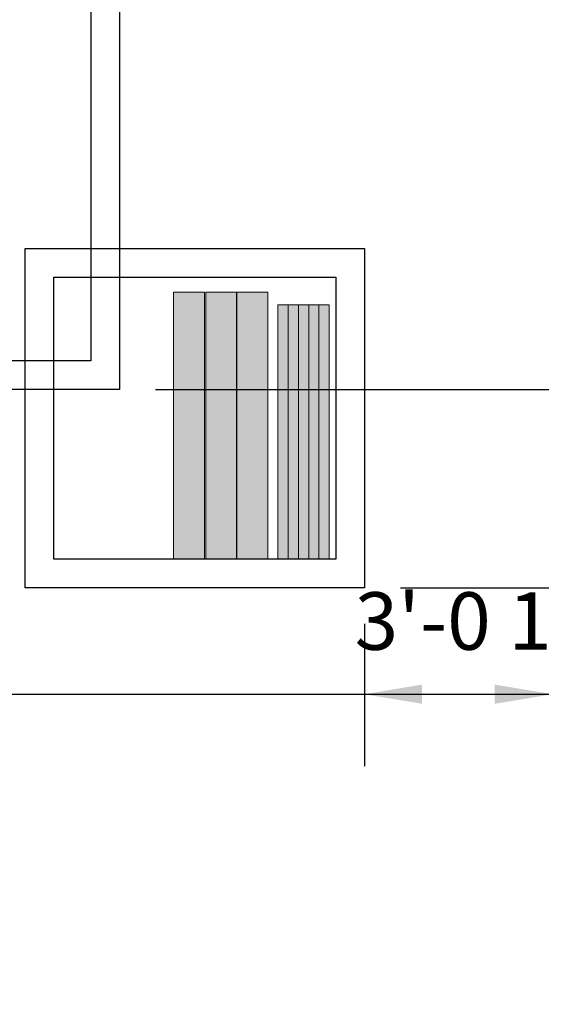
# Model space of a CAD drawing. Units: millimetres. Extents: x 7894 to 8038, y 6851 to 6951.
# Tile 5 of 49: x 7954.15 to 7963.22, y 6854.37 to 6871.49. Entities that reach past the tile are written whole.
import ezdxf

# ---------------------------------------------------------------- set-up
doc = ezdxf.new("R2010")
doc.units = ezdxf.units.MM
for name, color, linetype, lineweight in [('A-ANNO-DIMS', 2, 'Continuous', 18), ('A-FURN-BOOK', 8, 'Continuous', 13), ('A-FURN-CASE', 7, 'Continuous', 30)]:
    doc.layers.add(name, color=color, linetype=linetype, lineweight=lineweight)
doc.layers.add('A-FURN-PATT', color=32, linetype='Continuous', lineweight=9, true_color=0xcd6928)
doc.styles.get("Standard").update_dxf_attribs({"font": 'arial.ttf'})
doc.dimstyles.new('ISO-25', dxfattribs={"dimtxt": 1, "dimasz": 1, "dimexe": 1.25, "dimexo": 0.625, "dimtad": 1, "dimdec": 0, "dimlunit": 4, "dimtxsty": 'Standard', "dimcen": 2.5, "dimclrt": 1, "dimadec": 0, "dimazin": 0, "dimtfac": 1, "dimtdec": 0, "dimtmove": 0, "dimatfit": 3, "dimfxl": 1, "dimarcsym": 0})

# ---------------------------------------------------------------- blocks, each defined once
blk = doc.blocks.new('BOX-SHELF-SMALL-ELEV')
for points in [[(0, 5.9), (5.9, 5.9), (5.9, 0), (0, 0)], [(0.5, 5.4), (5.4, 5.4), (5.4, 0.5), (0.5, 0.5)]]:
    blk.add_lwpolyline(points, close=True)
blk = doc.blocks.new('*D36')
at = {"layer": 'A-ANNO-DIMS', "color": 0, "lineweight": -2, "transparency": 16777216}
for p, q in [((7980.836, 6877.959), (7980.836, 6858.512)), ((7944.487, 6864.436), (7944.487, 6858.512)), ((7945.487, 6859.762), (7979.836, 6859.762))]:
    blk.add_line(p, q, dxfattribs=at)
at = {"layer": 'A-ANNO-DIMS', "color": 0, "transparency": 16777216}
for points in [[(7945.487, 6859.929), (7945.487, 6859.596), (7944.487, 6859.762)], [(7979.836, 6859.929), (7979.836, 6859.596), (7980.836, 6859.762)]]:
    blk.add_solid(points, dxfattribs=at)
at = {"layer": 'Defpoints', "color": 0, "transparency": 16777216}
for p in [(7980.836, 6878.584), (7944.487, 6865.061), (7980.836, 6859.762)]:
    blk.add_point(p, dxfattribs=at)
at = {"layer": 'A-ANNO-DIMS', "color": 1, "transparency": 16777216, "insert": (7962.661, 6860.905), "char_height": 1, "attachment_point": 5}
blk.add_mtext('3\'-0 1/2"', dxfattribs=at)
blk = doc.blocks.new('*D37')
at = {"layer": 'A-ANNO-DIMS', "color": 0, "lineweight": -2, "transparency": 16777216}
for p, q in [((7954.92, 6887.903), (7941.389, 6887.903)), ((7942.639, 6862.61), (7942.639, 6886.903)), ((7953.623, 6861.61), (7941.389, 6861.61))]:
    blk.add_line(p, q, dxfattribs=at)
at = {"layer": 'A-ANNO-DIMS', "color": 0, "transparency": 16777216}
for points in [[(7942.472, 6886.903), (7942.806, 6886.903), (7942.639, 6887.903)], [(7942.472, 6862.61), (7942.806, 6862.61), (7942.639, 6861.61)]]:
    blk.add_solid(points, dxfattribs=at)
at = {"layer": 'Defpoints', "color": 0, "transparency": 16777216}
for p in [(7942.639, 6887.903), (7955.545, 6887.903), (7954.248, 6861.61)]:
    blk.add_point(p, dxfattribs=at)
at = {"layer": 'A-ANNO-DIMS', "color": 1, "transparency": 16777216, "insert": (7941.497, 6874.756), "char_height": 1, "attachment_point": 5, "rotation": 90}
blk.add_mtext('2\'-2 1/2"', dxfattribs=at)
blk = doc.blocks.new('*D41')
at = {"layer": 'A-ANNO-DIMS', "color": 0, "lineweight": -2, "transparency": 16777216}
for p, q in [((7982.683, 6865.722), (7982.683, 6870.631)), ((7964.039, 6864.722), (7983.933, 6864.722)), ((7982.683, 6861.61), (7982.683, 6864.722)), ((7960.773, 6861.61), (7983.933, 6861.61)), ((7982.683, 6860.61), (7982.683, 6859.61))]:
    blk.add_line(p, q, dxfattribs=at)
at = {"layer": 'A-ANNO-DIMS', "color": 0, "transparency": 16777216}
for points in [[(7982.517, 6865.722), (7982.85, 6865.722), (7982.683, 6864.722)], [(7982.517, 6860.61), (7982.85, 6860.61), (7982.683, 6861.61)]]:
    blk.add_solid(points, dxfattribs=at)
at = {"layer": 'Defpoints', "color": 0, "transparency": 16777216}
for p in [(7963.414, 6864.722), (7982.683, 6864.722), (7960.148, 6861.61)]:
    blk.add_point(p, dxfattribs=at)
at = {"layer": 'A-ANNO-DIMS', "color": 1, "transparency": 16777216, "insert": (7981.548, 6868.677), "char_height": 1, "attachment_point": 5, "rotation": 90}
blk.add_mtext('0\'-3"', dxfattribs=at)
blk = doc.blocks.new('*D44')
at = {"layer": 'A-ANNO-DIMS', "color": 0, "lineweight": -2, "transparency": 16777216}
for p, q in [((7963.414, 6864.097), (7963.414, 6858.512)), ((7960.148, 6860.985), (7960.148, 6858.512)), ((7961.148, 6859.762), (7962.414, 6859.762)), ((7963.414, 6859.762), (7970.652, 6859.762))]:
    blk.add_line(p, q, dxfattribs=at)
at = {"layer": 'A-ANNO-DIMS', "color": 0, "transparency": 16777216}
for points in [[(7961.148, 6859.929), (7961.148, 6859.596), (7960.148, 6859.762)], [(7962.414, 6859.929), (7962.414, 6859.596), (7963.414, 6859.762)]]:
    blk.add_solid(points, dxfattribs=at)
at = {"layer": 'Defpoints', "color": 0, "transparency": 16777216}
for p in [(7963.414, 6864.722), (7960.148, 6861.61), (7963.414, 6859.762)]:
    blk.add_point(p, dxfattribs=at)
at = {"layer": 'A-ANNO-DIMS', "color": 1, "transparency": 16777216, "insert": (7967.533, 6860.905), "char_height": 1, "attachment_point": 5}
blk.add_mtext('0\'-3 1/2"', dxfattribs=at)
blk = doc.blocks.new('*D45')
at = {"layer": 'A-ANNO-DIMS', "color": 0, "lineweight": -2, "transparency": 16777216}
for p, q in [((7956.512, 6865.061), (7983.933, 6865.061)), ((7982.683, 6864.061), (7982.683, 6862.61)), ((7960.773, 6861.61), (7983.933, 6861.61)), ((7982.683, 6861.61), (7982.683, 6854.371))]:
    blk.add_line(p, q, dxfattribs=at)
at = {"layer": 'A-ANNO-DIMS', "color": 0, "transparency": 16777216}
for points in [[(7982.517, 6864.061), (7982.85, 6864.061), (7982.683, 6865.061)], [(7982.517, 6862.61), (7982.85, 6862.61), (7982.683, 6861.61)]]:
    blk.add_solid(points, dxfattribs=at)
at = {"layer": 'Defpoints', "color": 0, "transparency": 16777216}
for p in [(7955.887, 6865.061), (7960.148, 6861.61), (7982.683, 6861.61)]:
    blk.add_point(p, dxfattribs=at)
at = {"layer": 'A-ANNO-DIMS', "color": 1, "transparency": 16777216, "insert": (7981.541, 6857.49), "char_height": 1, "attachment_point": 5, "rotation": 90}
blk.add_mtext('0\'-3 1/2"', dxfattribs=at)

msp = doc.modelspace()

# ---------------------------------------------------------------- hatches: boundary and pattern name
at = {"layer": 'A-FURN-PATT'}
h = msp.add_hatch(color=256, dxfattribs=at)
h.dxf.hatch_style = 1
h.paths.add_polyline_path([(7957.367, 6866.754), (7956.826, 6866.754), (7956.826, 6862.11), (7957.367, 6862.11)])
h.paths.add_polyline_path([(7957.925, 6866.754), (7957.386, 6866.754), (7957.386, 6862.11), (7957.925, 6862.11)])
h.paths.add_polyline_path([(7958.465, 6866.754), (7957.926, 6866.754), (7957.926, 6862.11), (7958.466, 6862.11)])
h = msp.add_hatch(color=256, dxfattribs=at)
h.dxf.hatch_style = 1
h.paths.add_polyline_path([(7958.999, 6866.533), (7958.821, 6866.533), (7958.821, 6862.11), (7958.999, 6862.11)])
h.paths.add_polyline_path([(7958.821, 6866.533), (7958.643, 6866.533), (7958.643, 6862.11), (7958.821, 6862.11)])
h = msp.add_hatch(color=256, dxfattribs=at)
h.dxf.hatch_style = 1
h.paths.add_polyline_path([(7959.534, 6866.533), (7959.356, 6866.533), (7959.356, 6862.11), (7959.534, 6862.11)])
h.paths.add_polyline_path([(7959.356, 6866.533), (7959.178, 6866.533), (7959.178, 6862.11), (7959.356, 6862.11)])
h.paths.add_polyline_path([(7959.178, 6866.533), (7958.999, 6866.533), (7958.999, 6862.11), (7959.178, 6862.11)])

# ---------------------------------------------------------------- linework, layer by layer
at = {"layer": 'A-FURN-BOOK'}
for p, q in [((7958.466, 6862.11), (7958.465, 6866.754)), ((7958.643, 6862.11), (7958.643, 6866.533)), ((7958.821, 6866.533), (7958.643, 6866.533)), ((7958.821, 6862.11), (7958.821, 6866.533)), ((7958.999, 6866.533), (7958.821, 6866.533)), ((7958.999, 6862.11), (7958.999, 6866.533)), ((7959.178, 6866.533), (7958.999, 6866.533)), ((7959.178, 6862.11), (7959.178, 6866.533)), ((7959.356, 6866.533), (7959.178, 6866.533)), ((7959.356, 6862.11), (7959.356, 6866.533)), ((7959.534, 6866.533), (7959.356, 6866.533)), ((7959.534, 6862.11), (7959.534, 6866.533)), ((7957.45, 6862.11), (7957.348, 6862.11)), ((7957.553, 6862.11), (7957.45, 6862.11)), ((7957.656, 6862.11), (7957.553, 6862.11)), ((7957.759, 6862.11), (7957.656, 6862.11)), ((7957.861, 6862.11), (7957.759, 6862.11)), ((7957.964, 6862.11), (7957.861, 6862.11)), ((7958.643, 6862.11), (7958.466, 6862.11)), ((7958.821, 6862.11), (7958.643, 6862.11)), ((7958.999, 6862.11), (7958.821, 6862.11)), ((7959.02, 6862.11), (7958.918, 6862.11)), ((7959.178, 6862.11), (7958.999, 6862.11)), ((7959.123, 6862.11), (7959.02, 6862.11)), ((7959.226, 6862.11), (7959.123, 6862.11)), ((7959.356, 6862.11), (7959.178, 6862.11)), ((7959.329, 6862.11), (7959.226, 6862.11)), ((7959.432, 6862.11), (7959.329, 6862.11)), ((7959.534, 6862.11), (7959.356, 6862.11)), ((7959.534, 6862.11), (7959.432, 6862.11))]:
    msp.add_line(p, q, dxfattribs=at)
for points in [[(7956.826, 6866.754), (7957.367, 6866.754), (7957.367, 6862.11), (7956.826, 6862.11)], [(7957.386, 6866.754), (7957.926, 6866.754), (7957.926, 6862.11), (7957.386, 6862.11)], [(7957.925, 6866.754), (7958.466, 6866.754), (7958.466, 6862.11), (7957.925, 6862.11)]]:
    msp.add_lwpolyline(points, close=True, dxfattribs=at)
at = {"layer": 'A-FURN-CASE'}
for points in [[(7944.487, 6876.461), (7955.887, 6876.461), (7955.887, 6865.061), (7944.487, 6865.061)], [(7944.987, 6875.961), (7955.387, 6875.961), (7955.387, 6865.561), (7944.987, 6865.561)]]:
    msp.add_lwpolyline(points, close=True, dxfattribs=at)

# ---------------------------------------------------------------- block references
msp.add_blockref('BOX-SHELF-SMALL-ELEV', (7954.248, 6861.61), dxfattribs=at)

# ---------------------------------------------------------------- dimensions: what is measured, and where the dimension line sits
at = {"layer": 'A-ANNO-DIMS'}
for base, p1, p2, picture, middle in [((7942.639, 6887.903), (7954.248, 6861.61), (7955.545, 6887.903), '*D37', (7941.497, 6874.756)), ((7982.683, 6864.722), (7960.148, 6861.61), (7963.414, 6864.722), '*D41', (7981.548, 6868.677)), ((7982.683, 6861.61), (7955.887, 6865.061), (7960.148, 6861.61), '*D45', (7981.541, 6857.49))]:
    dim = msp.add_linear_dim(base=base, p1=p1, p2=p2, angle=90, dimstyle='ISO-25', override={"dimdec": 1, "dimlfac": 1, "dimrnd": 0, "dimzin": 1, "dimdsep": 46, "dimlunit": 4, "dimfrac": 2}, dxfattribs=at)
    dim.commit()
    dim.dimension.update_dxf_attribs({"geometry": picture, "text_midpoint": middle})
for base, p1, p2, picture, middle in [((7980.836, 6859.762), (7944.487, 6865.061), (7980.836, 6878.584), '*D36', (7962.661, 6860.905)), ((7963.414, 6859.762), (7960.148, 6861.61), (7963.414, 6864.722), '*D44', (7967.533, 6860.905))]:
    dim = msp.add_linear_dim(base=base, p1=p1, p2=p2, dimstyle='ISO-25', override={"dimdec": 1, "dimlfac": 1, "dimrnd": 0, "dimzin": 1, "dimdsep": 46, "dimlunit": 4, "dimfrac": 2}, dxfattribs=at)
    dim.commit()
    dim.dimension.update_dxf_attribs({"geometry": picture, "text_midpoint": middle})

doc.saveas('drawing.dxf')
